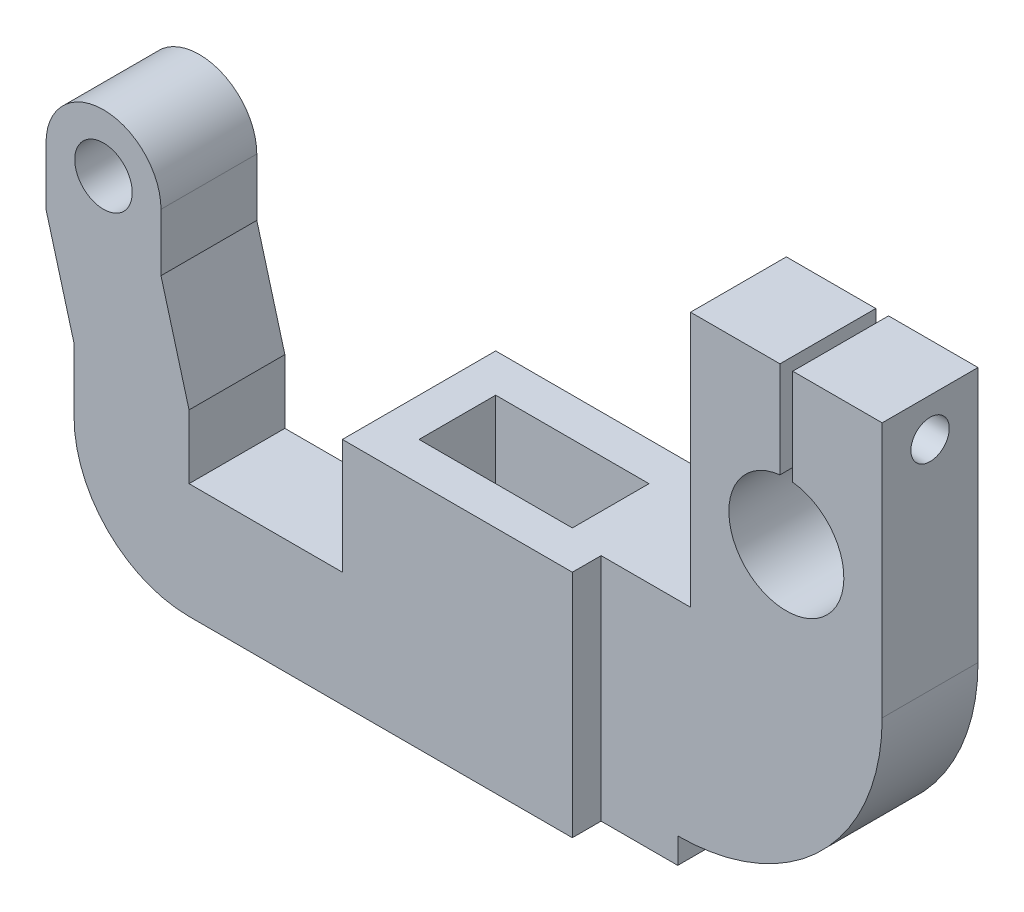
ISO-10303-21;
HEADER;
FILE_DESCRIPTION(('STEP AP214'),'2;1');
FILE_NAME('part.step','',(''),(''),'','','');
FILE_SCHEMA(('AUTOMOTIVE_DESIGN { 1 0 10303 214 1 1 1 1 }'));
ENDSEC;
DATA;
#1=APPLICATION_CONTEXT('core data for automotive mechanical design processes');
#2=APPLICATION_PROTOCOL_DEFINITION('international standard','automotive_design',2000,#1);
#3=PRODUCT_CONTEXT('',#1,'mechanical');
#4=PRODUCT('Part','Part','',(#3));
#5=PRODUCT_RELATED_PRODUCT_CATEGORY('part','',(#4));
#6=PRODUCT_DEFINITION_FORMATION('','',#4);
#7=PRODUCT_DEFINITION_CONTEXT('part definition',#1,'design');
#8=PRODUCT_DEFINITION('design','',#6,#7);
#9=PRODUCT_DEFINITION_SHAPE('','',#8);
#10=(LENGTH_UNIT() NAMED_UNIT(*) SI_UNIT(.MILLI.,.METRE.));
#11=(NAMED_UNIT(*) PLANE_ANGLE_UNIT() SI_UNIT($,.RADIAN.));
#12=(NAMED_UNIT(*) SI_UNIT($,.STERADIAN.) SOLID_ANGLE_UNIT());
#13=UNCERTAINTY_MEASURE_WITH_UNIT(LENGTH_MEASURE(1.E-05),#10,'distance_accuracy_value','');
#14=(GEOMETRIC_REPRESENTATION_CONTEXT(3) GLOBAL_UNCERTAINTY_ASSIGNED_CONTEXT((#13)) GLOBAL_UNIT_ASSIGNED_CONTEXT((#10,
#11,#12)) REPRESENTATION_CONTEXT('',''));
#15=CARTESIAN_POINT('',(0.,0.,0.));
#16=DIRECTION('',(0.,0.,1.));
#17=DIRECTION('',(1.,0.,0.));
#18=AXIS2_PLACEMENT_3D('',#15,#16,#17);
#19=CARTESIAN_POINT('',(-18.,36.,-12.));
#20=DIRECTION('',(1.,0.,0.));
#21=DIRECTION('',(0.,0.,-1.));
#22=AXIS2_PLACEMENT_3D('',#19,#20,#21);
#23=PLANE('',#22);
#24=DIRECTION('',(0.,0.,-1.));
#25=VECTOR('',#24,1.);
#26=CARTESIAN_POINT('',(-18.,18.,12.));
#27=LINE('',#26,#25);
#28=CARTESIAN_POINT('',(-18.,18.,12.));
#29=VERTEX_POINT('',#28);
#30=CARTESIAN_POINT('',(-18.,18.,-3.));
#31=VERTEX_POINT('',#30);
#32=EDGE_CURVE('E54',#29,#31,#27,.T.);
#33=ORIENTED_EDGE('',*,*,#32,.F.);
#34=DIRECTION('',(0.,-1.,0.));
#35=VECTOR('',#34,1.);
#36=CARTESIAN_POINT('',(-18.,36.,12.));
#37=LINE('',#36,#35);
#38=CARTESIAN_POINT('',(-18.,36.,12.));
#39=VERTEX_POINT('',#38);
#40=EDGE_CURVE('E480',#39,#29,#37,.T.);
#41=ORIENTED_EDGE('',*,*,#40,.F.);
#42=DIRECTION('',(0.,0.,1.));
#43=VECTOR('',#42,1.);
#44=CARTESIAN_POINT('',(-18.,36.,-12.));
#45=LINE('',#44,#43);
#46=CARTESIAN_POINT('',(-18.,36.,-12.));
#47=VERTEX_POINT('',#46);
#48=EDGE_CURVE('E459',#47,#39,#45,.T.);
#49=ORIENTED_EDGE('',*,*,#48,.F.);
#50=DIRECTION('',(0.,-1.,0.));
#51=VECTOR('',#50,1.);
#52=CARTESIAN_POINT('',(-18.,36.,-12.));
#53=LINE('',#52,#51);
#54=CARTESIAN_POINT('',(-18.,0.,-12.));
#55=VERTEX_POINT('',#54);
#56=EDGE_CURVE('E479',#47,#55,#53,.T.);
#57=ORIENTED_EDGE('',*,*,#56,.T.);
#58=DIRECTION('',(0.,0.,1.));
#59=VECTOR('',#58,1.);
#60=CARTESIAN_POINT('',(-18.,0.,-12.));
#61=LINE('',#60,#59);
#62=CARTESIAN_POINT('',(-18.,0.,-3.));
#63=VERTEX_POINT('',#62);
#64=EDGE_CURVE('E468',#55,#63,#61,.T.);
#65=ORIENTED_EDGE('',*,*,#64,.T.);
#66=DIRECTION('',(0.,1.,0.));
#67=VECTOR('',#66,1.);
#68=CARTESIAN_POINT('',(-18.,0.,-3.));
#69=LINE('',#68,#67);
#70=EDGE_CURVE('E324',#63,#31,#69,.T.);
#71=ORIENTED_EDGE('',*,*,#70,.T.);
#72=EDGE_LOOP('',(#33,#41,#49,#57,#65,#71));
#73=FACE_BOUND('',#72,.T.);
#74=ADVANCED_FACE('F39',(#73),#23,.F.);
#75=CARTESIAN_POINT('',(0.,76.,0.));
#76=DIRECTION('',(0.,-1.,0.));
#77=DIRECTION('',(0.,0.,-1.));
#78=AXIS2_PLACEMENT_3D('',#75,#76,#77);
#79=PLANE('',#78);
#80=DIRECTION('',(-1.,0.,0.));
#81=VECTOR('',#80,1.);
#82=CARTESIAN_POINT('',(62.,76.,-7.5));
#83=LINE('',#82,#81);
#84=CARTESIAN_POINT('',(62.,76.,-7.5));
#85=VERTEX_POINT('',#84);
#86=CARTESIAN_POINT('',(48.,76.,-7.5));
#87=VERTEX_POINT('',#86);
#88=EDGE_CURVE('E364',#85,#87,#83,.T.);
#89=ORIENTED_EDGE('',*,*,#88,.T.);
#90=DIRECTION('',(0.,0.,1.));
#91=VECTOR('',#90,1.);
#92=CARTESIAN_POINT('',(48.,76.,0.));
#93=LINE('',#92,#91);
#94=CARTESIAN_POINT('',(48.,76.,7.5));
#95=VERTEX_POINT('',#94);
#96=EDGE_CURVE('E11',#87,#95,#93,.T.);
#97=ORIENTED_EDGE('',*,*,#96,.T.);
#98=DIRECTION('',(1.,0.,0.));
#99=VECTOR('',#98,1.);
#100=CARTESIAN_POINT('',(62.,76.,7.5));
#101=LINE('',#100,#99);
#102=CARTESIAN_POINT('',(62.,76.,7.5));
#103=VERTEX_POINT('',#102);
#104=EDGE_CURVE('E367',#95,#103,#101,.T.);
#105=ORIENTED_EDGE('',*,*,#104,.T.);
#106=DIRECTION('',(0.,0.,-1.));
#107=VECTOR('',#106,1.);
#108=CARTESIAN_POINT('',(62.,76.,-7.5));
#109=LINE('',#108,#107);
#110=EDGE_CURVE('E359',#103,#85,#109,.T.);
#111=ORIENTED_EDGE('',*,*,#110,.T.);
#112=EDGE_LOOP('',(#89,#97,#105,#111));
#113=FACE_BOUND('',#112,.T.);
#114=ADVANCED_FACE('F512',(#113),#79,.F.);
#115=CARTESIAN_POINT('',(30.,0.,-7.5));
#116=DIRECTION('',(1.,0.,0.));
#117=DIRECTION('',(0.,0.,-1.));
#118=AXIS2_PLACEMENT_3D('',#115,#116,#117);
#119=PLANE('',#118);
#120=DIRECTION('',(0.,1.,0.));
#121=VECTOR('',#120,1.);
#122=CARTESIAN_POINT('',(30.,0.,-7.5));
#123=LINE('',#122,#121);
#124=CARTESIAN_POINT('',(30.,0.,-7.5));
#125=VERTEX_POINT('',#124);
#126=CARTESIAN_POINT('',(30.,4.,-7.5));
#127=VERTEX_POINT('',#126);
#128=EDGE_CURVE('E413',#125,#127,#123,.T.);
#129=ORIENTED_EDGE('',*,*,#128,.T.);
#130=DIRECTION('',(0.,0.,1.));
#131=VECTOR('',#130,1.);
#132=CARTESIAN_POINT('',(30.,4.,-7.5));
#133=LINE('',#132,#131);
#134=CARTESIAN_POINT('',(30.,4.,7.5));
#135=VERTEX_POINT('',#134);
#136=EDGE_CURVE('E388',#127,#135,#133,.T.);
#137=ORIENTED_EDGE('',*,*,#136,.T.);
#138=DIRECTION('',(0.,1.,0.));
#139=VECTOR('',#138,1.);
#140=CARTESIAN_POINT('',(30.,0.,7.5));
#141=LINE('',#140,#139);
#142=CARTESIAN_POINT('',(30.,0.,7.5));
#143=VERTEX_POINT('',#142);
#144=EDGE_CURVE('E419',#143,#135,#141,.T.);
#145=ORIENTED_EDGE('',*,*,#144,.F.);
#146=DIRECTION('',(0.,0.,-1.));
#147=VECTOR('',#146,1.);
#148=CARTESIAN_POINT('',(30.,0.,-7.5));
#149=LINE('',#148,#147);
#150=EDGE_CURVE('E402',#143,#125,#149,.T.);
#151=ORIENTED_EDGE('',*,*,#150,.T.);
#152=EDGE_LOOP('',(#129,#137,#145,#151));
#153=FACE_BOUND('',#152,.T.);
#154=ADVANCED_FACE('F525',(#153),#119,.T.);
#155=CARTESIAN_POINT('',(18.,36.,-12.));
#156=DIRECTION('',(-1.,0.,0.));
#157=DIRECTION('',(0.,0.,1.));
#158=AXIS2_PLACEMENT_3D('',#155,#156,#157);
#159=PLANE('',#158);
#160=DIRECTION('',(0.,1.,0.));
#161=VECTOR('',#160,1.);
#162=CARTESIAN_POINT('',(18.,0.,-7.5));
#163=LINE('',#162,#161);
#164=CARTESIAN_POINT('',(18.,0.,-7.5));
#165=VERTEX_POINT('',#164);
#166=CARTESIAN_POINT('',(18.,36.,-7.5));
#167=VERTEX_POINT('',#166);
#168=EDGE_CURVE('E408',#165,#167,#163,.T.);
#169=ORIENTED_EDGE('',*,*,#168,.F.);
#170=DIRECTION('',(0.,0.,-1.));
#171=VECTOR('',#170,1.);
#172=CARTESIAN_POINT('',(18.,0.,-12.));
#173=LINE('',#172,#171);
#174=CARTESIAN_POINT('',(18.,0.,-12.));
#175=VERTEX_POINT('',#174);
#176=EDGE_CURVE('E450',#165,#175,#173,.T.);
#177=ORIENTED_EDGE('',*,*,#176,.T.);
#178=DIRECTION('',(0.,-1.,0.));
#179=VECTOR('',#178,1.);
#180=CARTESIAN_POINT('',(18.,36.,-12.));
#181=LINE('',#180,#179);
#182=CARTESIAN_POINT('',(18.,36.,-12.));
#183=VERTEX_POINT('',#182);
#184=EDGE_CURVE('E482',#183,#175,#181,.T.);
#185=ORIENTED_EDGE('',*,*,#184,.F.);
#186=DIRECTION('',(0.,0.,-1.));
#187=VECTOR('',#186,1.);
#188=CARTESIAN_POINT('',(18.,36.,-12.));
#189=LINE('',#188,#187);
#190=EDGE_CURVE('E457',#167,#183,#189,.T.);
#191=ORIENTED_EDGE('',*,*,#190,.F.);
#192=EDGE_LOOP('',(#169,#177,#185,#191));
#193=FACE_BOUND('',#192,.T.);
#194=ADVANCED_FACE('F534',(#193),#159,.F.);
#195=CARTESIAN_POINT('',(18.,0.,12.));
#196=VERTEX_POINT('',#195);
#197=CARTESIAN_POINT('',(18.,0.,7.5));
#198=VERTEX_POINT('',#197);
#199=EDGE_CURVE('E461',#196,#198,#173,.T.);
#200=ORIENTED_EDGE('',*,*,#199,.T.);
#201=DIRECTION('',(0.,1.,0.));
#202=VECTOR('',#201,1.);
#203=CARTESIAN_POINT('',(18.,0.,7.5));
#204=LINE('',#203,#202);
#205=CARTESIAN_POINT('',(18.,36.,7.5));
#206=VERTEX_POINT('',#205);
#207=EDGE_CURVE('E410',#198,#206,#204,.T.);
#208=ORIENTED_EDGE('',*,*,#207,.T.);
#209=CARTESIAN_POINT('',(18.,36.,12.));
#210=VERTEX_POINT('',#209);
#211=EDGE_CURVE('E451',#210,#206,#189,.T.);
#212=ORIENTED_EDGE('',*,*,#211,.F.);
#213=DIRECTION('',(0.,-1.,0.));
#214=VECTOR('',#213,1.);
#215=CARTESIAN_POINT('',(18.,36.,12.));
#216=LINE('',#215,#214);
#217=EDGE_CURVE('E465',#210,#196,#216,.T.);
#218=ORIENTED_EDGE('',*,*,#217,.T.);
#219=EDGE_LOOP('',(#200,#208,#212,#218));
#220=FACE_BOUND('',#219,.T.);
#221=ADVANCED_FACE('F41',(#220),#159,.F.);
#222=CARTESIAN_POINT('',(-18.,36.,-12.));
#223=DIRECTION('',(0.,0.,1.));
#224=DIRECTION('',(1.,0.,0.));
#225=AXIS2_PLACEMENT_3D('',#222,#223,#224);
#226=PLANE('',#225);
#227=DIRECTION('',(-1.,0.,0.));
#228=VECTOR('',#227,1.);
#229=CARTESIAN_POINT('',(-18.,0.,-12.));
#230=LINE('',#229,#228);
#231=EDGE_CURVE('E466',#175,#55,#230,.T.);
#232=ORIENTED_EDGE('',*,*,#231,.T.);
#233=ORIENTED_EDGE('',*,*,#56,.F.);
#234=DIRECTION('',(-1.,0.,0.));
#235=VECTOR('',#234,1.);
#236=CARTESIAN_POINT('',(-18.,36.,-12.));
#237=LINE('',#236,#235);
#238=EDGE_CURVE('E460',#183,#47,#237,.T.);
#239=ORIENTED_EDGE('',*,*,#238,.F.);
#240=ORIENTED_EDGE('',*,*,#184,.T.);
#241=EDGE_LOOP('',(#232,#233,#239,#240));
#242=FACE_BOUND('',#241,.T.);
#243=ADVANCED_FACE('F545',(#242),#226,.F.);
#244=CARTESIAN_POINT('',(-18.,36.,12.));
#245=DIRECTION('',(0.,0.,-1.));
#246=DIRECTION('',(-1.,0.,0.));
#247=AXIS2_PLACEMENT_3D('',#244,#245,#246);
#248=PLANE('',#247);
#249=DIRECTION('',(1.,0.,0.));
#250=VECTOR('',#249,1.);
#251=CARTESIAN_POINT('',(-18.,0.,12.));
#252=LINE('',#251,#250);
#253=CARTESIAN_POINT('',(-42.,0.,12.));
#254=VERTEX_POINT('',#253);
#255=EDGE_CURVE('E474',#254,#196,#252,.T.);
#256=ORIENTED_EDGE('',*,*,#255,.T.);
#257=ORIENTED_EDGE('',*,*,#217,.F.);
#258=DIRECTION('',(1.,0.,0.));
#259=VECTOR('',#258,1.);
#260=CARTESIAN_POINT('',(-18.,36.,12.));
#261=LINE('',#260,#259);
#262=EDGE_CURVE('E464',#39,#210,#261,.T.);
#263=ORIENTED_EDGE('',*,*,#262,.F.);
#264=ORIENTED_EDGE('',*,*,#40,.T.);
#265=DIRECTION('',(1.,0.,0.));
#266=VECTOR('',#265,1.);
#267=CARTESIAN_POINT('',(-18.,18.,12.));
#268=LINE('',#267,#266);
#269=CARTESIAN_POINT('',(-42.,18.,12.));
#270=VERTEX_POINT('',#269);
#271=EDGE_CURVE('E322',#270,#29,#268,.T.);
#272=ORIENTED_EDGE('',*,*,#271,.F.);
#273=DIRECTION('',(0.,1.,0.));
#274=VECTOR('',#273,1.);
#275=CARTESIAN_POINT('',(-42.,18.,12.));
#276=LINE('',#275,#274);
#277=CARTESIAN_POINT('',(-42.,28.,12.));
#278=VERTEX_POINT('',#277);
#279=EDGE_CURVE('E293',#270,#278,#276,.T.);
#280=ORIENTED_EDGE('',*,*,#279,.T.);
#281=DIRECTION('',(-0.264769001023054,0.964311866616425,0.));
#282=VECTOR('',#281,1.);
#283=CARTESIAN_POINT('',(-42.,28.,12.));
#284=LINE('',#283,#282);
#285=CARTESIAN_POINT('',(-46.3930850205475,44.,12.));
#286=VERTEX_POINT('',#285);
#287=EDGE_CURVE('E282',#278,#286,#284,.T.);
#288=ORIENTED_EDGE('',*,*,#287,.T.);
#289=DIRECTION('',(0.,1.,0.));
#290=VECTOR('',#289,1.);
#291=CARTESIAN_POINT('',(-46.3930850205475,53.,12.));
#292=LINE('',#291,#290);
#293=CARTESIAN_POINT('',(-46.3930850205475,53.,12.));
#294=VERTEX_POINT('',#293);
#295=EDGE_CURVE('E274',#286,#294,#292,.T.);
#296=ORIENTED_EDGE('',*,*,#295,.T.);
#297=CARTESIAN_POINT('',(-55.3930850205475,53.,12.));
#298=DIRECTION('',(0.,0.,1.));
#299=DIRECTION('',(1.,0.,0.));
#300=AXIS2_PLACEMENT_3D('',#297,#298,#299);
#301=CIRCLE('',#300,9.);
#302=CARTESIAN_POINT('',(-64.3930850205475,53.,12.));
#303=VERTEX_POINT('',#302);
#304=EDGE_CURVE('E244',#294,#303,#301,.T.);
#305=ORIENTED_EDGE('',*,*,#304,.T.);
#306=DIRECTION('',(0.,-1.,0.));
#307=VECTOR('',#306,1.);
#308=CARTESIAN_POINT('',(-64.3930850205475,44.,12.));
#309=LINE('',#308,#307);
#310=CARTESIAN_POINT('',(-64.3930850205475,44.,12.));
#311=VERTEX_POINT('',#310);
#312=EDGE_CURVE('E264',#303,#311,#309,.T.);
#313=ORIENTED_EDGE('',*,*,#312,.T.);
#314=DIRECTION('',(0.264769001023054,-0.964311866616425,0.));
#315=VECTOR('',#314,1.);
#316=CARTESIAN_POINT('',(-60.,28.,12.));
#317=LINE('',#316,#315);
#318=CARTESIAN_POINT('',(-60.,28.,12.));
#319=VERTEX_POINT('',#318);
#320=EDGE_CURVE('E279',#311,#319,#317,.T.);
#321=ORIENTED_EDGE('',*,*,#320,.T.);
#322=DIRECTION('',(0.,-1.,0.));
#323=VECTOR('',#322,1.);
#324=CARTESIAN_POINT('',(-60.,18.,12.));
#325=LINE('',#324,#323);
#326=CARTESIAN_POINT('',(-60.,18.,12.));
#327=VERTEX_POINT('',#326);
#328=EDGE_CURVE('E304',#319,#327,#325,.T.);
#329=ORIENTED_EDGE('',*,*,#328,.T.);
#330=CARTESIAN_POINT('',(-42.,18.,12.));
#331=DIRECTION('',(0.,0.,1.));
#332=DIRECTION('',(1.,0.,0.));
#333=AXIS2_PLACEMENT_3D('',#330,#331,#332);
#334=CIRCLE('',#333,18.);
#335=EDGE_CURVE('E300',#327,#254,#334,.T.);
#336=ORIENTED_EDGE('',*,*,#335,.T.);
#337=EDGE_LOOP('',(#256,#257,#263,#264,#272,#280,#288,#296,#305,#313,#321,#329,#336));
#338=FACE_BOUND('',#337,.T.);
#339=CARTESIAN_POINT('',(-55.3930850205475,53.,12.));
#340=DIRECTION('',(0.,0.,1.));
#341=DIRECTION('',(1.,0.,0.));
#342=AXIS2_PLACEMENT_3D('',#339,#340,#341);
#343=CIRCLE('',#342,4.5);
#344=CARTESIAN_POINT('',(-50.8930850205475,53.,12.));
#345=VERTEX_POINT('',#344);
#346=EDGE_CURVE('E266',#345,#345,#343,.T.);
#347=ORIENTED_EDGE('',*,*,#346,.F.);
#348=EDGE_LOOP('',(#347));
#349=FACE_BOUND('',#348,.T.);
#350=ADVANCED_FACE('F553',(#338,#349),#248,.F.);
#351=CARTESIAN_POINT('',(0.,36.,0.));
#352=DIRECTION('',(0.,1.,0.));
#353=DIRECTION('',(0.,0.,1.));
#354=AXIS2_PLACEMENT_3D('',#351,#352,#353);
#355=PLANE('',#354);
#356=DIRECTION('',(0.,0.,1.));
#357=VECTOR('',#356,1.);
#358=CARTESIAN_POINT('',(32.,36.,-7.5));
#359=LINE('',#358,#357);
#360=CARTESIAN_POINT('',(32.,36.,-7.5));
#361=VERTEX_POINT('',#360);
#362=CARTESIAN_POINT('',(32.,36.,7.5));
#363=VERTEX_POINT('',#362);
#364=EDGE_CURVE('E360',#361,#363,#359,.T.);
#365=ORIENTED_EDGE('',*,*,#364,.F.);
#366=DIRECTION('',(-1.,0.,0.));
#367=VECTOR('',#366,1.);
#368=CARTESIAN_POINT('',(18.,36.,-7.5));
#369=LINE('',#368,#367);
#370=EDGE_CURVE('E405',#361,#167,#369,.T.);
#371=ORIENTED_EDGE('',*,*,#370,.T.);
#372=ORIENTED_EDGE('',*,*,#190,.T.);
#373=ORIENTED_EDGE('',*,*,#238,.T.);
#374=ORIENTED_EDGE('',*,*,#48,.T.);
#375=ORIENTED_EDGE('',*,*,#262,.T.);
#376=ORIENTED_EDGE('',*,*,#211,.T.);
#377=DIRECTION('',(1.,0.,0.));
#378=VECTOR('',#377,1.);
#379=CARTESIAN_POINT('',(18.,36.,7.5));
#380=LINE('',#379,#378);
#381=EDGE_CURVE('E394',#206,#363,#380,.T.);
#382=ORIENTED_EDGE('',*,*,#381,.T.);
#383=EDGE_LOOP('',(#365,#371,#372,#373,#374,#375,#376,#382));
#384=FACE_BOUND('',#383,.T.);
#385=DIRECTION('',(0.,0.,-1.));
#386=VECTOR('',#385,1.);
#387=CARTESIAN_POINT('',(12.,36.,-6.));
#388=LINE('',#387,#386);
#389=CARTESIAN_POINT('',(12.,36.,6.));
#390=VERTEX_POINT('',#389);
#391=CARTESIAN_POINT('',(12.,36.,-6.));
#392=VERTEX_POINT('',#391);
#393=EDGE_CURVE('E412',#390,#392,#388,.T.);
#394=ORIENTED_EDGE('',*,*,#393,.F.);
#395=DIRECTION('',(1.,0.,0.));
#396=VECTOR('',#395,1.);
#397=CARTESIAN_POINT('',(-12.,36.,6.));
#398=LINE('',#397,#396);
#399=CARTESIAN_POINT('',(-12.,36.,6.));
#400=VERTEX_POINT('',#399);
#401=EDGE_CURVE('E428',#400,#390,#398,.T.);
#402=ORIENTED_EDGE('',*,*,#401,.F.);
#403=DIRECTION('',(0.,0.,1.));
#404=VECTOR('',#403,1.);
#405=CARTESIAN_POINT('',(-12.,36.,-6.));
#406=LINE('',#405,#404);
#407=CARTESIAN_POINT('',(-12.,36.,-6.));
#408=VERTEX_POINT('',#407);
#409=EDGE_CURVE('E439',#408,#400,#406,.T.);
#410=ORIENTED_EDGE('',*,*,#409,.F.);
#411=DIRECTION('',(-1.,0.,0.));
#412=VECTOR('',#411,1.);
#413=CARTESIAN_POINT('',(-12.,36.,-6.));
#414=LINE('',#413,#412);
#415=EDGE_CURVE('E440',#392,#408,#414,.T.);
#416=ORIENTED_EDGE('',*,*,#415,.F.);
#417=EDGE_LOOP('',(#394,#402,#410,#416));
#418=FACE_BOUND('',#417,.T.);
#419=ADVANCED_FACE('F539',(#384,#418),#355,.T.);
#420=CARTESIAN_POINT('',(0.,0.,0.));
#421=DIRECTION('',(0.,1.,0.));
#422=DIRECTION('',(0.,0.,1.));
#423=AXIS2_PLACEMENT_3D('',#420,#421,#422);
#424=PLANE('',#423);
#425=DIRECTION('',(1.,0.,0.));
#426=VECTOR('',#425,1.);
#427=CARTESIAN_POINT('',(-12.,0.,6.));
#428=LINE('',#427,#426);
#429=CARTESIAN_POINT('',(-12.,0.,6.));
#430=VERTEX_POINT('',#429);
#431=CARTESIAN_POINT('',(12.,0.,6.));
#432=VERTEX_POINT('',#431);
#433=EDGE_CURVE('E435',#430,#432,#428,.T.);
#434=ORIENTED_EDGE('',*,*,#433,.T.);
#435=DIRECTION('',(0.,0.,-1.));
#436=VECTOR('',#435,1.);
#437=CARTESIAN_POINT('',(12.,0.,-6.));
#438=LINE('',#437,#436);
#439=CARTESIAN_POINT('',(12.,0.,-6.));
#440=VERTEX_POINT('',#439);
#441=EDGE_CURVE('E422',#432,#440,#438,.T.);
#442=ORIENTED_EDGE('',*,*,#441,.T.);
#443=DIRECTION('',(-1.,0.,0.));
#444=VECTOR('',#443,1.);
#445=CARTESIAN_POINT('',(-12.,0.,-6.));
#446=LINE('',#445,#444);
#447=CARTESIAN_POINT('',(-12.,0.,-6.));
#448=VERTEX_POINT('',#447);
#449=EDGE_CURVE('E424',#440,#448,#446,.T.);
#450=ORIENTED_EDGE('',*,*,#449,.T.);
#451=DIRECTION('',(0.,0.,1.));
#452=VECTOR('',#451,1.);
#453=CARTESIAN_POINT('',(-12.,0.,-6.));
#454=LINE('',#453,#452);
#455=EDGE_CURVE('E429',#448,#430,#454,.T.);
#456=ORIENTED_EDGE('',*,*,#455,.T.);
#457=EDGE_LOOP('',(#434,#442,#450,#456));
#458=FACE_BOUND('',#457,.T.);
#459=ORIENTED_EDGE('',*,*,#199,.F.);
#460=ORIENTED_EDGE('',*,*,#255,.F.);
#461=DIRECTION('',(0.,0.,1.));
#462=VECTOR('',#461,1.);
#463=CARTESIAN_POINT('',(-42.,0.,12.));
#464=LINE('',#463,#462);
#465=CARTESIAN_POINT('',(-42.,0.,-3.));
#466=VERTEX_POINT('',#465);
#467=EDGE_CURVE('E318',#466,#254,#464,.T.);
#468=ORIENTED_EDGE('',*,*,#467,.F.);
#469=DIRECTION('',(-1.,0.,0.));
#470=VECTOR('',#469,1.);
#471=CARTESIAN_POINT('',(-18.,0.,-3.));
#472=LINE('',#471,#470);
#473=EDGE_CURVE('E320',#63,#466,#472,.T.);
#474=ORIENTED_EDGE('',*,*,#473,.F.);
#475=ORIENTED_EDGE('',*,*,#64,.F.);
#476=ORIENTED_EDGE('',*,*,#231,.F.);
#477=ORIENTED_EDGE('',*,*,#176,.F.);
#478=DIRECTION('',(-1.,0.,0.));
#479=VECTOR('',#478,1.);
#480=CARTESIAN_POINT('',(18.,0.,-7.5));
#481=LINE('',#480,#479);
#482=EDGE_CURVE('E403',#125,#165,#481,.T.);
#483=ORIENTED_EDGE('',*,*,#482,.F.);
#484=ORIENTED_EDGE('',*,*,#150,.F.);
#485=DIRECTION('',(1.,0.,0.));
#486=VECTOR('',#485,1.);
#487=CARTESIAN_POINT('',(18.,0.,7.5));
#488=LINE('',#487,#486);
#489=EDGE_CURVE('E397',#198,#143,#488,.T.);
#490=ORIENTED_EDGE('',*,*,#489,.F.);
#491=EDGE_LOOP('',(#459,#460,#468,#474,#475,#476,#477,#483,#484,#490));
#492=FACE_BOUND('',#491,.T.);
#493=ADVANCED_FACE('F530',(#458,#492),#424,.F.);
#494=CARTESIAN_POINT('',(12.,0.,-6.));
#495=DIRECTION('',(1.,0.,0.));
#496=DIRECTION('',(0.,0.,-1.));
#497=AXIS2_PLACEMENT_3D('',#494,#495,#496);
#498=PLANE('',#497);
#499=ORIENTED_EDGE('',*,*,#393,.T.);
#500=DIRECTION('',(0.,1.,0.));
#501=VECTOR('',#500,1.);
#502=CARTESIAN_POINT('',(12.,0.,-6.));
#503=LINE('',#502,#501);
#504=EDGE_CURVE('E434',#440,#392,#503,.T.);
#505=ORIENTED_EDGE('',*,*,#504,.F.);
#506=ORIENTED_EDGE('',*,*,#441,.F.);
#507=DIRECTION('',(0.,1.,0.));
#508=VECTOR('',#507,1.);
#509=CARTESIAN_POINT('',(12.,0.,6.));
#510=LINE('',#509,#508);
#511=EDGE_CURVE('E444',#432,#390,#510,.T.);
#512=ORIENTED_EDGE('',*,*,#511,.T.);
#513=EDGE_LOOP('',(#499,#505,#506,#512));
#514=FACE_BOUND('',#513,.T.);
#515=ADVANCED_FACE('F622',(#514),#498,.F.);
#516=CARTESIAN_POINT('',(-12.,0.,6.));
#517=DIRECTION('',(0.,0.,1.));
#518=DIRECTION('',(1.,0.,0.));
#519=AXIS2_PLACEMENT_3D('',#516,#517,#518);
#520=PLANE('',#519);
#521=ORIENTED_EDGE('',*,*,#401,.T.);
#522=ORIENTED_EDGE('',*,*,#511,.F.);
#523=ORIENTED_EDGE('',*,*,#433,.F.);
#524=DIRECTION('',(0.,1.,0.));
#525=VECTOR('',#524,1.);
#526=CARTESIAN_POINT('',(-12.,0.,6.));
#527=LINE('',#526,#525);
#528=EDGE_CURVE('E449',#430,#400,#527,.T.);
#529=ORIENTED_EDGE('',*,*,#528,.T.);
#530=EDGE_LOOP('',(#521,#522,#523,#529));
#531=FACE_BOUND('',#530,.T.);
#532=ADVANCED_FACE('F623',(#531),#520,.F.);
#533=CARTESIAN_POINT('',(-12.,0.,-6.));
#534=DIRECTION('',(-1.,0.,0.));
#535=DIRECTION('',(0.,0.,1.));
#536=AXIS2_PLACEMENT_3D('',#533,#534,#535);
#537=PLANE('',#536);
#538=ORIENTED_EDGE('',*,*,#409,.T.);
#539=ORIENTED_EDGE('',*,*,#528,.F.);
#540=ORIENTED_EDGE('',*,*,#455,.F.);
#541=DIRECTION('',(0.,1.,0.));
#542=VECTOR('',#541,1.);
#543=CARTESIAN_POINT('',(-12.,0.,-6.));
#544=LINE('',#543,#542);
#545=EDGE_CURVE('E448',#448,#408,#544,.T.);
#546=ORIENTED_EDGE('',*,*,#545,.T.);
#547=EDGE_LOOP('',(#538,#539,#540,#546));
#548=FACE_BOUND('',#547,.T.);
#549=ADVANCED_FACE('F624',(#548),#537,.F.);
#550=CARTESIAN_POINT('',(-12.,0.,-6.));
#551=DIRECTION('',(0.,0.,-1.));
#552=DIRECTION('',(-1.,0.,0.));
#553=AXIS2_PLACEMENT_3D('',#550,#551,#552);
#554=PLANE('',#553);
#555=ORIENTED_EDGE('',*,*,#415,.T.);
#556=ORIENTED_EDGE('',*,*,#545,.F.);
#557=ORIENTED_EDGE('',*,*,#449,.F.);
#558=ORIENTED_EDGE('',*,*,#504,.T.);
#559=EDGE_LOOP('',(#555,#556,#557,#558));
#560=FACE_BOUND('',#559,.T.);
#561=ADVANCED_FACE('F627',(#560),#554,.F.);
#562=CARTESIAN_POINT('',(18.,0.,-7.5));
#563=DIRECTION('',(0.,0.,-1.));
#564=DIRECTION('',(-1.,0.,0.));
#565=AXIS2_PLACEMENT_3D('',#562,#563,#564);
#566=PLANE('',#565);
#567=DIRECTION('',(0.,-1.,0.));
#568=VECTOR('',#567,1.);
#569=CARTESIAN_POINT('',(48.,0.,-7.5));
#570=LINE('',#569,#568);
#571=CARTESIAN_POINT('',(48.,60.9442719099992,-7.5));
#572=VERTEX_POINT('',#571);
#573=EDGE_CURVE('E351',#87,#572,#570,.T.);
#574=ORIENTED_EDGE('',*,*,#573,.F.);
#575=ORIENTED_EDGE('',*,*,#88,.F.);
#576=DIRECTION('',(0.,-1.,0.));
#577=VECTOR('',#576,1.);
#578=CARTESIAN_POINT('',(62.,76.,-7.5));
#579=LINE('',#578,#577);
#580=CARTESIAN_POINT('',(62.,36.,-7.5));
#581=VERTEX_POINT('',#580);
#582=EDGE_CURVE('E381',#85,#581,#579,.T.);
#583=ORIENTED_EDGE('',*,*,#582,.T.);
#584=CARTESIAN_POINT('',(30.,36.,-7.5));
#585=DIRECTION('',(0.,0.,1.));
#586=DIRECTION('',(1.,0.,0.));
#587=AXIS2_PLACEMENT_3D('',#584,#585,#586);
#588=CIRCLE('',#587,32.);
#589=EDGE_CURVE('E389',#127,#581,#588,.T.);
#590=ORIENTED_EDGE('',*,*,#589,.F.);
#591=ORIENTED_EDGE('',*,*,#128,.F.);
#592=ORIENTED_EDGE('',*,*,#482,.T.);
#593=ORIENTED_EDGE('',*,*,#168,.T.);
#594=ORIENTED_EDGE('',*,*,#370,.F.);
#595=DIRECTION('',(0.,-1.,0.));
#596=VECTOR('',#595,1.);
#597=CARTESIAN_POINT('',(32.,76.,-7.5));
#598=LINE('',#597,#596);
#599=CARTESIAN_POINT('',(32.,76.,-7.5));
#600=VERTEX_POINT('',#599);
#601=EDGE_CURVE('E382',#600,#361,#598,.T.);
#602=ORIENTED_EDGE('',*,*,#601,.F.);
#603=CARTESIAN_POINT('',(46.,76.,-7.5));
#604=VERTEX_POINT('',#603);
#605=EDGE_CURVE('E361',#604,#600,#83,.T.);
#606=ORIENTED_EDGE('',*,*,#605,.F.);
#607=DIRECTION('',(0.,1.,0.));
#608=VECTOR('',#607,1.);
#609=CARTESIAN_POINT('',(46.,0.,-7.5));
#610=LINE('',#609,#608);
#611=CARTESIAN_POINT('',(46.,60.9442719099992,-7.5));
#612=VERTEX_POINT('',#611);
#613=EDGE_CURVE('E64',#612,#604,#610,.T.);
#614=ORIENTED_EDGE('',*,*,#613,.F.);
#615=CARTESIAN_POINT('',(47.,52.,-7.5));
#616=DIRECTION('',(0.,0.,-1.));
#617=DIRECTION('',(-1.,0.,0.));
#618=AXIS2_PLACEMENT_3D('',#615,#616,#617);
#619=CIRCLE('',#618,9.00000000000001);
#620=EDGE_CURVE('E357',#572,#612,#619,.T.);
#621=ORIENTED_EDGE('',*,*,#620,.F.);
#622=EDGE_LOOP('',(#574,#575,#583,#590,#591,#592,#593,#594,#602,#606,#614,#621));
#623=FACE_BOUND('',#622,.T.);
#624=ADVANCED_FACE('F494',(#623),#566,.T.);
#625=CARTESIAN_POINT('',(18.,0.,7.5));
#626=DIRECTION('',(0.,0.,1.));
#627=DIRECTION('',(1.,0.,0.));
#628=AXIS2_PLACEMENT_3D('',#625,#626,#627);
#629=PLANE('',#628);
#630=DIRECTION('',(0.,1.,0.));
#631=VECTOR('',#630,1.);
#632=CARTESIAN_POINT('',(48.,76.,7.5));
#633=LINE('',#632,#631);
#634=CARTESIAN_POINT('',(48.,60.9442719099992,7.5));
#635=VERTEX_POINT('',#634);
#636=EDGE_CURVE('E347',#635,#95,#633,.T.);
#637=ORIENTED_EDGE('',*,*,#636,.F.);
#638=CARTESIAN_POINT('',(47.,52.,7.5));
#639=DIRECTION('',(0.,0.,1.));
#640=DIRECTION('',(1.,0.,0.));
#641=AXIS2_PLACEMENT_3D('',#638,#639,#640);
#642=CIRCLE('',#641,9.00000000000001);
#643=CARTESIAN_POINT('',(46.,60.9442719099992,7.5));
#644=VERTEX_POINT('',#643);
#645=EDGE_CURVE('E343',#644,#635,#642,.T.);
#646=ORIENTED_EDGE('',*,*,#645,.F.);
#647=DIRECTION('',(0.,-1.,0.));
#648=VECTOR('',#647,1.);
#649=CARTESIAN_POINT('',(46.,76.,7.5));
#650=LINE('',#649,#648);
#651=CARTESIAN_POINT('',(46.,76.,7.5));
#652=VERTEX_POINT('',#651);
#653=EDGE_CURVE('E345',#652,#644,#650,.T.);
#654=ORIENTED_EDGE('',*,*,#653,.F.);
#655=CARTESIAN_POINT('',(32.,76.,7.5));
#656=VERTEX_POINT('',#655);
#657=EDGE_CURVE('E369',#656,#652,#101,.T.);
#658=ORIENTED_EDGE('',*,*,#657,.F.);
#659=DIRECTION('',(0.,-1.,0.));
#660=VECTOR('',#659,1.);
#661=CARTESIAN_POINT('',(32.,76.,7.5));
#662=LINE('',#661,#660);
#663=EDGE_CURVE('E377',#656,#363,#662,.T.);
#664=ORIENTED_EDGE('',*,*,#663,.T.);
#665=ORIENTED_EDGE('',*,*,#381,.F.);
#666=ORIENTED_EDGE('',*,*,#207,.F.);
#667=ORIENTED_EDGE('',*,*,#489,.T.);
#668=ORIENTED_EDGE('',*,*,#144,.T.);
#669=CARTESIAN_POINT('',(30.,36.,7.5));
#670=DIRECTION('',(0.,0.,1.));
#671=DIRECTION('',(1.,0.,0.));
#672=AXIS2_PLACEMENT_3D('',#669,#670,#671);
#673=CIRCLE('',#672,32.);
#674=CARTESIAN_POINT('',(62.,36.,7.5));
#675=VERTEX_POINT('',#674);
#676=EDGE_CURVE('E390',#135,#675,#673,.T.);
#677=ORIENTED_EDGE('',*,*,#676,.T.);
#678=DIRECTION('',(0.,-1.,0.));
#679=VECTOR('',#678,1.);
#680=CARTESIAN_POINT('',(62.,76.,7.5));
#681=LINE('',#680,#679);
#682=EDGE_CURVE('E373',#103,#675,#681,.T.);
#683=ORIENTED_EDGE('',*,*,#682,.F.);
#684=ORIENTED_EDGE('',*,*,#104,.F.);
#685=EDGE_LOOP('',(#637,#646,#654,#658,#664,#665,#666,#667,#668,#677,#683,#684));
#686=FACE_BOUND('',#685,.T.);
#687=ADVANCED_FACE('F503',(#686),#629,.T.);
#688=CARTESIAN_POINT('',(30.,36.,-7.5));
#689=DIRECTION('',(0.,0.,1.));
#690=DIRECTION('',(1.,0.,0.));
#691=AXIS2_PLACEMENT_3D('',#688,#689,#690);
#692=CYLINDRICAL_SURFACE('',#691,32.);
#693=ORIENTED_EDGE('',*,*,#676,.F.);
#694=ORIENTED_EDGE('',*,*,#136,.F.);
#695=ORIENTED_EDGE('',*,*,#589,.T.);
#696=DIRECTION('',(0.,0.,1.));
#697=VECTOR('',#696,1.);
#698=CARTESIAN_POINT('',(62.,36.,-7.5));
#699=LINE('',#698,#697);
#700=EDGE_CURVE('E392',#581,#675,#699,.T.);
#701=ORIENTED_EDGE('',*,*,#700,.T.);
#702=EDGE_LOOP('',(#693,#694,#695,#701));
#703=FACE_BOUND('',#702,.T.);
#704=ADVANCED_FACE('F619',(#703),#692,.T.);
#705=CARTESIAN_POINT('',(62.,76.,-7.5));
#706=DIRECTION('',(-1.,0.,0.));
#707=DIRECTION('',(0.,0.,1.));
#708=AXIS2_PLACEMENT_3D('',#705,#706,#707);
#709=PLANE('',#708);
#710=CARTESIAN_POINT('',(62.,70.,0.));
#711=DIRECTION('',(1.,0.,0.));
#712=DIRECTION('',(0.,0.,-1.));
#713=AXIS2_PLACEMENT_3D('',#710,#711,#712);
#714=CIRCLE('',#713,3.);
#715=CARTESIAN_POINT('',(62.,70.,-3.));
#716=VERTEX_POINT('',#715);
#717=EDGE_CURVE('E332',#716,#716,#714,.T.);
#718=ORIENTED_EDGE('',*,*,#717,.F.);
#719=EDGE_LOOP('',(#718));
#720=FACE_BOUND('',#719,.T.);
#721=ORIENTED_EDGE('',*,*,#700,.F.);
#722=ORIENTED_EDGE('',*,*,#582,.F.);
#723=ORIENTED_EDGE('',*,*,#110,.F.);
#724=ORIENTED_EDGE('',*,*,#682,.T.);
#725=EDGE_LOOP('',(#721,#722,#723,#724));
#726=FACE_BOUND('',#725,.T.);
#727=ADVANCED_FACE('F519',(#720,#726),#709,.F.);
#728=CARTESIAN_POINT('',(32.,76.,-7.5));
#729=DIRECTION('',(1.,0.,0.));
#730=DIRECTION('',(0.,0.,-1.));
#731=AXIS2_PLACEMENT_3D('',#728,#729,#730);
#732=PLANE('',#731);
#733=CARTESIAN_POINT('',(32.,70.,0.));
#734=DIRECTION('',(1.,0.,0.));
#735=DIRECTION('',(0.,0.,-1.));
#736=AXIS2_PLACEMENT_3D('',#733,#734,#735);
#737=CIRCLE('',#736,3.);
#738=CARTESIAN_POINT('',(32.,70.,-3.));
#739=VERTEX_POINT('',#738);
#740=EDGE_CURVE('E339',#739,#739,#737,.T.);
#741=ORIENTED_EDGE('',*,*,#740,.T.);
#742=EDGE_LOOP('',(#741));
#743=FACE_BOUND('',#742,.T.);
#744=ORIENTED_EDGE('',*,*,#364,.T.);
#745=ORIENTED_EDGE('',*,*,#663,.F.);
#746=DIRECTION('',(0.,0.,1.));
#747=VECTOR('',#746,1.);
#748=CARTESIAN_POINT('',(32.,76.,-7.5));
#749=LINE('',#748,#747);
#750=EDGE_CURVE('E370',#600,#656,#749,.T.);
#751=ORIENTED_EDGE('',*,*,#750,.F.);
#752=ORIENTED_EDGE('',*,*,#601,.T.);
#753=EDGE_LOOP('',(#744,#745,#751,#752));
#754=FACE_BOUND('',#753,.T.);
#755=ADVANCED_FACE('F499',(#743,#754),#732,.F.);
#756=ORIENTED_EDGE('',*,*,#657,.T.);
#757=DIRECTION('',(0.,0.,-1.));
#758=VECTOR('',#757,1.);
#759=CARTESIAN_POINT('',(46.,76.,0.));
#760=LINE('',#759,#758);
#761=EDGE_CURVE('E48',#652,#604,#760,.T.);
#762=ORIENTED_EDGE('',*,*,#761,.T.);
#763=ORIENTED_EDGE('',*,*,#605,.T.);
#764=ORIENTED_EDGE('',*,*,#750,.T.);
#765=EDGE_LOOP('',(#756,#762,#763,#764));
#766=FACE_BOUND('',#765,.T.);
#767=ADVANCED_FACE('F486',(#766),#79,.F.);
#768=CARTESIAN_POINT('',(48.,76.,-12.));
#769=DIRECTION('',(1.,0.,0.));
#770=DIRECTION('',(0.,0.,-1.));
#771=AXIS2_PLACEMENT_3D('',#768,#769,#770);
#772=PLANE('',#771);
#773=CARTESIAN_POINT('',(48.,70.,0.));
#774=DIRECTION('',(1.,0.,0.));
#775=DIRECTION('',(0.,0.,-1.));
#776=AXIS2_PLACEMENT_3D('',#773,#774,#775);
#777=CIRCLE('',#776,3.);
#778=CARTESIAN_POINT('',(48.,70.,-3.));
#779=VERTEX_POINT('',#778);
#780=EDGE_CURVE('E337',#779,#779,#777,.T.);
#781=ORIENTED_EDGE('',*,*,#780,.T.);
#782=EDGE_LOOP('',(#781));
#783=FACE_BOUND('',#782,.T.);
#784=ORIENTED_EDGE('',*,*,#573,.T.);
#785=DIRECTION('',(0.,0.,1.));
#786=VECTOR('',#785,1.);
#787=CARTESIAN_POINT('',(48.,60.9442719099992,-12.));
#788=LINE('',#787,#786);
#789=EDGE_CURVE('E353',#572,#635,#788,.T.);
#790=ORIENTED_EDGE('',*,*,#789,.T.);
#791=ORIENTED_EDGE('',*,*,#636,.T.);
#792=ORIENTED_EDGE('',*,*,#96,.F.);
#793=EDGE_LOOP('',(#784,#790,#791,#792));
#794=FACE_BOUND('',#793,.T.);
#795=ADVANCED_FACE('F770',(#783,#794),#772,.F.);
#796=CARTESIAN_POINT('',(47.,52.,-12.));
#797=DIRECTION('',(0.,0.,1.));
#798=DIRECTION('',(1.,0.,0.));
#799=AXIS2_PLACEMENT_3D('',#796,#797,#798);
#800=CYLINDRICAL_SURFACE('',#799,9.00000000000001);
#801=ORIENTED_EDGE('',*,*,#620,.T.);
#802=DIRECTION('',(0.,0.,1.));
#803=VECTOR('',#802,1.);
#804=CARTESIAN_POINT('',(46.,60.9442719099992,-12.));
#805=LINE('',#804,#803);
#806=EDGE_CURVE('E349',#612,#644,#805,.T.);
#807=ORIENTED_EDGE('',*,*,#806,.T.);
#808=ORIENTED_EDGE('',*,*,#645,.T.);
#809=ORIENTED_EDGE('',*,*,#789,.F.);
#810=EDGE_LOOP('',(#801,#807,#808,#809));
#811=FACE_BOUND('',#810,.T.);
#812=ADVANCED_FACE('F510',(#811),#800,.F.);
#813=CARTESIAN_POINT('',(46.,76.,-12.));
#814=DIRECTION('',(-1.,0.,0.));
#815=DIRECTION('',(0.,0.,1.));
#816=AXIS2_PLACEMENT_3D('',#813,#814,#815);
#817=PLANE('',#816);
#818=CARTESIAN_POINT('',(46.,70.,0.));
#819=DIRECTION('',(-1.,0.,0.));
#820=DIRECTION('',(0.,0.,1.));
#821=AXIS2_PLACEMENT_3D('',#818,#819,#820);
#822=CIRCLE('',#821,3.);
#823=CARTESIAN_POINT('',(46.,70.,3.));
#824=VERTEX_POINT('',#823);
#825=EDGE_CURVE('E43',#824,#824,#822,.T.);
#826=ORIENTED_EDGE('',*,*,#825,.T.);
#827=EDGE_LOOP('',(#826));
#828=FACE_BOUND('',#827,.T.);
#829=ORIENTED_EDGE('',*,*,#613,.T.);
#830=ORIENTED_EDGE('',*,*,#761,.F.);
#831=ORIENTED_EDGE('',*,*,#653,.T.);
#832=ORIENTED_EDGE('',*,*,#806,.F.);
#833=EDGE_LOOP('',(#829,#830,#831,#832));
#834=FACE_BOUND('',#833,.T.);
#835=ADVANCED_FACE('F504',(#828,#834),#817,.F.);
#836=CARTESIAN_POINT('',(-18.,70.,0.));
#837=DIRECTION('',(1.,0.,0.));
#838=DIRECTION('',(0.,0.,-1.));
#839=AXIS2_PLACEMENT_3D('',#836,#837,#838);
#840=CYLINDRICAL_SURFACE('',#839,3.);
#841=ORIENTED_EDGE('',*,*,#825,.F.);
#842=EDGE_LOOP('',(#841));
#843=FACE_BOUND('',#842,.T.);
#844=ORIENTED_EDGE('',*,*,#740,.F.);
#845=EDGE_LOOP('',(#844));
#846=FACE_BOUND('',#845,.T.);
#847=ADVANCED_FACE('F761',(#843,#846),#840,.F.);
#848=ORIENTED_EDGE('',*,*,#717,.T.);
#849=EDGE_LOOP('',(#848));
#850=FACE_BOUND('',#849,.T.);
#851=ORIENTED_EDGE('',*,*,#780,.F.);
#852=EDGE_LOOP('',(#851));
#853=FACE_BOUND('',#852,.T.);
#854=ADVANCED_FACE('F676',(#850,#853),#840,.F.);
#855=CARTESIAN_POINT('',(-18.,0.,-3.));
#856=DIRECTION('',(0.,0.,-1.));
#857=DIRECTION('',(-1.,0.,0.));
#858=AXIS2_PLACEMENT_3D('',#855,#856,#857);
#859=PLANE('',#858);
#860=DIRECTION('',(-1.,0.,0.));
#861=VECTOR('',#860,1.);
#862=CARTESIAN_POINT('',(-18.,18.,-3.));
#863=LINE('',#862,#861);
#864=CARTESIAN_POINT('',(-42.,18.,-3.));
#865=VERTEX_POINT('',#864);
#866=EDGE_CURVE('E323',#31,#865,#863,.T.);
#867=ORIENTED_EDGE('',*,*,#866,.F.);
#868=ORIENTED_EDGE('',*,*,#70,.F.);
#869=ORIENTED_EDGE('',*,*,#473,.T.);
#870=CARTESIAN_POINT('',(-42.,18.,-3.));
#871=DIRECTION('',(0.,0.,1.));
#872=DIRECTION('',(1.,0.,0.));
#873=AXIS2_PLACEMENT_3D('',#870,#871,#872);
#874=CIRCLE('',#873,18.);
#875=CARTESIAN_POINT('',(-60.,18.,-3.));
#876=VERTEX_POINT('',#875);
#877=EDGE_CURVE('E297',#876,#466,#874,.T.);
#878=ORIENTED_EDGE('',*,*,#877,.F.);
#879=DIRECTION('',(0.,-1.,0.));
#880=VECTOR('',#879,1.);
#881=CARTESIAN_POINT('',(-60.,18.,-3.));
#882=LINE('',#881,#880);
#883=CARTESIAN_POINT('',(-60.,28.,-3.));
#884=VERTEX_POINT('',#883);
#885=EDGE_CURVE('E298',#884,#876,#882,.T.);
#886=ORIENTED_EDGE('',*,*,#885,.F.);
#887=DIRECTION('',(0.264769001023054,-0.964311866616425,0.));
#888=VECTOR('',#887,1.);
#889=CARTESIAN_POINT('',(-60.,28.,-3.));
#890=LINE('',#889,#888);
#891=CARTESIAN_POINT('',(-64.3930850205475,44.,-3.));
#892=VERTEX_POINT('',#891);
#893=EDGE_CURVE('E278',#892,#884,#890,.T.);
#894=ORIENTED_EDGE('',*,*,#893,.F.);
#895=DIRECTION('',(0.,-1.,0.));
#896=VECTOR('',#895,1.);
#897=CARTESIAN_POINT('',(-64.3930850205475,44.,-3.));
#898=LINE('',#897,#896);
#899=CARTESIAN_POINT('',(-64.3930850205475,53.,-3.));
#900=VERTEX_POINT('',#899);
#901=EDGE_CURVE('E252',#900,#892,#898,.T.);
#902=ORIENTED_EDGE('',*,*,#901,.F.);
#903=CARTESIAN_POINT('',(-55.3930850205475,53.,-3.));
#904=DIRECTION('',(0.,0.,1.));
#905=DIRECTION('',(1.,0.,0.));
#906=AXIS2_PLACEMENT_3D('',#903,#904,#905);
#907=CIRCLE('',#906,9.);
#908=CARTESIAN_POINT('',(-46.3930850205475,53.,-3.));
#909=VERTEX_POINT('',#908);
#910=EDGE_CURVE('E245',#909,#900,#907,.T.);
#911=ORIENTED_EDGE('',*,*,#910,.F.);
#912=DIRECTION('',(0.,1.,0.));
#913=VECTOR('',#912,1.);
#914=CARTESIAN_POINT('',(-46.3930850205475,53.,-3.));
#915=LINE('',#914,#913);
#916=CARTESIAN_POINT('',(-46.3930850205475,44.,-3.));
#917=VERTEX_POINT('',#916);
#918=EDGE_CURVE('E259',#917,#909,#915,.T.);
#919=ORIENTED_EDGE('',*,*,#918,.F.);
#920=DIRECTION('',(-0.264769001023054,0.964311866616425,0.));
#921=VECTOR('',#920,1.);
#922=CARTESIAN_POINT('',(-42.,28.,-3.));
#923=LINE('',#922,#921);
#924=CARTESIAN_POINT('',(-42.,28.,-3.));
#925=VERTEX_POINT('',#924);
#926=EDGE_CURVE('E285',#925,#917,#923,.T.);
#927=ORIENTED_EDGE('',*,*,#926,.F.);
#928=DIRECTION('',(0.,1.,0.));
#929=VECTOR('',#928,1.);
#930=CARTESIAN_POINT('',(-42.,0.,-3.));
#931=LINE('',#930,#929);
#932=EDGE_CURVE('E291',#865,#925,#931,.T.);
#933=ORIENTED_EDGE('',*,*,#932,.F.);
#934=EDGE_LOOP('',(#867,#868,#869,#878,#886,#894,#902,#911,#919,#927,#933));
#935=FACE_BOUND('',#934,.T.);
#936=CARTESIAN_POINT('',(-55.3930850205475,53.,-3.));
#937=DIRECTION('',(0.,0.,1.));
#938=DIRECTION('',(1.,0.,0.));
#939=AXIS2_PLACEMENT_3D('',#936,#937,#938);
#940=CIRCLE('',#939,4.5);
#941=CARTESIAN_POINT('',(-50.8930850205475,53.,-3.));
#942=VERTEX_POINT('',#941);
#943=EDGE_CURVE('E277',#942,#942,#940,.T.);
#944=ORIENTED_EDGE('',*,*,#943,.T.);
#945=EDGE_LOOP('',(#944));
#946=FACE_BOUND('',#945,.T.);
#947=ADVANCED_FACE('F253',(#935,#946),#859,.T.);
#948=CARTESIAN_POINT('',(0.,18.,0.));
#949=DIRECTION('',(0.,1.,0.));
#950=DIRECTION('',(0.,0.,1.));
#951=AXIS2_PLACEMENT_3D('',#948,#949,#950);
#952=PLANE('',#951);
#953=ORIENTED_EDGE('',*,*,#32,.T.);
#954=ORIENTED_EDGE('',*,*,#866,.T.);
#955=DIRECTION('',(0.,0.,1.));
#956=VECTOR('',#955,1.);
#957=CARTESIAN_POINT('',(-42.,18.,12.));
#958=LINE('',#957,#956);
#959=EDGE_CURVE('E330',#865,#270,#958,.T.);
#960=ORIENTED_EDGE('',*,*,#959,.T.);
#961=ORIENTED_EDGE('',*,*,#271,.T.);
#962=EDGE_LOOP('',(#953,#954,#960,#961));
#963=FACE_BOUND('',#962,.T.);
#964=ADVANCED_FACE('F563',(#963),#952,.T.);
#965=CARTESIAN_POINT('',(-42.,18.,-3.));
#966=DIRECTION('',(1.,0.,0.));
#967=DIRECTION('',(0.,0.,-1.));
#968=AXIS2_PLACEMENT_3D('',#965,#966,#967);
#969=PLANE('',#968);
#970=ORIENTED_EDGE('',*,*,#959,.F.);
#971=ORIENTED_EDGE('',*,*,#932,.T.);
#972=DIRECTION('',(0.,0.,1.));
#973=VECTOR('',#972,1.);
#974=CARTESIAN_POINT('',(-42.,28.,-3.));
#975=LINE('',#974,#973);
#976=EDGE_CURVE('E305',#925,#278,#975,.T.);
#977=ORIENTED_EDGE('',*,*,#976,.T.);
#978=ORIENTED_EDGE('',*,*,#279,.F.);
#979=EDGE_LOOP('',(#970,#971,#977,#978));
#980=FACE_BOUND('',#979,.T.);
#981=ADVANCED_FACE('F564',(#980),#969,.T.);
#982=CARTESIAN_POINT('',(-42.,18.,-3.));
#983=DIRECTION('',(0.,0.,1.));
#984=DIRECTION('',(1.,0.,0.));
#985=AXIS2_PLACEMENT_3D('',#982,#983,#984);
#986=CYLINDRICAL_SURFACE('',#985,18.);
#987=ORIENTED_EDGE('',*,*,#335,.F.);
#988=DIRECTION('',(0.,0.,1.));
#989=VECTOR('',#988,1.);
#990=CARTESIAN_POINT('',(-60.,18.,-3.));
#991=LINE('',#990,#989);
#992=EDGE_CURVE('E309',#876,#327,#991,.T.);
#993=ORIENTED_EDGE('',*,*,#992,.F.);
#994=ORIENTED_EDGE('',*,*,#877,.T.);
#995=ORIENTED_EDGE('',*,*,#467,.T.);
#996=EDGE_LOOP('',(#987,#993,#994,#995));
#997=FACE_BOUND('',#996,.T.);
#998=ADVANCED_FACE('F580',(#997),#986,.T.);
#999=CARTESIAN_POINT('',(-60.,18.,-3.));
#1000=DIRECTION('',(-1.,0.,0.));
#1001=DIRECTION('',(0.,0.,1.));
#1002=AXIS2_PLACEMENT_3D('',#999,#1000,#1001);
#1003=PLANE('',#1002);
#1004=ORIENTED_EDGE('',*,*,#328,.F.);
#1005=DIRECTION('',(0.,0.,1.));
#1006=VECTOR('',#1005,1.);
#1007=CARTESIAN_POINT('',(-60.,28.,-3.));
#1008=LINE('',#1007,#1006);
#1009=EDGE_CURVE('E315',#884,#319,#1008,.T.);
#1010=ORIENTED_EDGE('',*,*,#1009,.F.);
#1011=ORIENTED_EDGE('',*,*,#885,.T.);
#1012=ORIENTED_EDGE('',*,*,#992,.T.);
#1013=EDGE_LOOP('',(#1004,#1010,#1011,#1012));
#1014=FACE_BOUND('',#1013,.T.);
#1015=ADVANCED_FACE('F577',(#1014),#1003,.T.);
#1016=CARTESIAN_POINT('',(-60.,28.,-3.));
#1017=DIRECTION('',(-0.964311866616425,-0.264769001023053,0.));
#1018=DIRECTION('',(0.264769001023054,-0.964311866616425,0.));
#1019=AXIS2_PLACEMENT_3D('',#1016,#1017,#1018);
#1020=PLANE('',#1019);
#1021=ORIENTED_EDGE('',*,*,#320,.F.);
#1022=DIRECTION('',(0.,0.,1.));
#1023=VECTOR('',#1022,1.);
#1024=CARTESIAN_POINT('',(-64.3930850205475,44.,-3.));
#1025=LINE('',#1024,#1023);
#1026=EDGE_CURVE('E287',#892,#311,#1025,.T.);
#1027=ORIENTED_EDGE('',*,*,#1026,.F.);
#1028=ORIENTED_EDGE('',*,*,#893,.T.);
#1029=ORIENTED_EDGE('',*,*,#1009,.T.);
#1030=EDGE_LOOP('',(#1021,#1027,#1028,#1029));
#1031=FACE_BOUND('',#1030,.T.);
#1032=ADVANCED_FACE('F575',(#1031),#1020,.T.);
#1033=CARTESIAN_POINT('',(-42.,28.,-3.));
#1034=DIRECTION('',(0.964311866616425,0.264769001023053,0.));
#1035=DIRECTION('',(-0.264769001023054,0.964311866616425,0.));
#1036=AXIS2_PLACEMENT_3D('',#1033,#1034,#1035);
#1037=PLANE('',#1036);
#1038=ORIENTED_EDGE('',*,*,#287,.F.);
#1039=ORIENTED_EDGE('',*,*,#976,.F.);
#1040=ORIENTED_EDGE('',*,*,#926,.T.);
#1041=DIRECTION('',(0.,0.,1.));
#1042=VECTOR('',#1041,1.);
#1043=CARTESIAN_POINT('',(-46.3930850205475,44.,-3.));
#1044=LINE('',#1043,#1042);
#1045=EDGE_CURVE('E263',#917,#286,#1044,.T.);
#1046=ORIENTED_EDGE('',*,*,#1045,.T.);
#1047=EDGE_LOOP('',(#1038,#1039,#1040,#1046));
#1048=FACE_BOUND('',#1047,.T.);
#1049=ADVANCED_FACE('F570',(#1048),#1037,.T.);
#1050=CARTESIAN_POINT('',(-64.3930850205475,44.,-3.));
#1051=DIRECTION('',(-1.,0.,0.));
#1052=DIRECTION('',(0.,0.,1.));
#1053=AXIS2_PLACEMENT_3D('',#1050,#1051,#1052);
#1054=PLANE('',#1053);
#1055=ORIENTED_EDGE('',*,*,#312,.F.);
#1056=DIRECTION('',(0.,0.,1.));
#1057=VECTOR('',#1056,1.);
#1058=CARTESIAN_POINT('',(-64.3930850205475,53.,-3.));
#1059=LINE('',#1058,#1057);
#1060=EDGE_CURVE('E249',#900,#303,#1059,.T.);
#1061=ORIENTED_EDGE('',*,*,#1060,.F.);
#1062=ORIENTED_EDGE('',*,*,#901,.T.);
#1063=ORIENTED_EDGE('',*,*,#1026,.T.);
#1064=EDGE_LOOP('',(#1055,#1061,#1062,#1063));
#1065=FACE_BOUND('',#1064,.T.);
#1066=ADVANCED_FACE('F569',(#1065),#1054,.T.);
#1067=CARTESIAN_POINT('',(-55.3930850205475,53.,-3.));
#1068=DIRECTION('',(0.,0.,1.));
#1069=DIRECTION('',(1.,0.,0.));
#1070=AXIS2_PLACEMENT_3D('',#1067,#1068,#1069);
#1071=CYLINDRICAL_SURFACE('',#1070,9.);
#1072=ORIENTED_EDGE('',*,*,#304,.F.);
#1073=DIRECTION('',(0.,0.,1.));
#1074=VECTOR('',#1073,1.);
#1075=CARTESIAN_POINT('',(-46.3930850205475,53.,-3.));
#1076=LINE('',#1075,#1074);
#1077=EDGE_CURVE('E237',#909,#294,#1076,.T.);
#1078=ORIENTED_EDGE('',*,*,#1077,.F.);
#1079=ORIENTED_EDGE('',*,*,#910,.T.);
#1080=ORIENTED_EDGE('',*,*,#1060,.T.);
#1081=EDGE_LOOP('',(#1072,#1078,#1079,#1080));
#1082=FACE_BOUND('',#1081,.T.);
#1083=ADVANCED_FACE('F241',(#1082),#1071,.T.);
#1084=CARTESIAN_POINT('',(-46.3930850205475,53.,-3.));
#1085=DIRECTION('',(1.,0.,0.));
#1086=DIRECTION('',(0.,0.,-1.));
#1087=AXIS2_PLACEMENT_3D('',#1084,#1085,#1086);
#1088=PLANE('',#1087);
#1089=ORIENTED_EDGE('',*,*,#295,.F.);
#1090=ORIENTED_EDGE('',*,*,#1045,.F.);
#1091=ORIENTED_EDGE('',*,*,#918,.T.);
#1092=ORIENTED_EDGE('',*,*,#1077,.T.);
#1093=EDGE_LOOP('',(#1089,#1090,#1091,#1092));
#1094=FACE_BOUND('',#1093,.T.);
#1095=ADVANCED_FACE('F262',(#1094),#1088,.T.);
#1096=CARTESIAN_POINT('',(-55.3930850205475,53.,-3.));
#1097=DIRECTION('',(0.,0.,1.));
#1098=DIRECTION('',(1.,0.,0.));
#1099=AXIS2_PLACEMENT_3D('',#1096,#1097,#1098);
#1100=CYLINDRICAL_SURFACE('',#1099,4.5);
#1101=ORIENTED_EDGE('',*,*,#943,.F.);
#1102=EDGE_LOOP('',(#1101));
#1103=FACE_BOUND('',#1102,.T.);
#1104=ORIENTED_EDGE('',*,*,#346,.T.);
#1105=EDGE_LOOP('',(#1104));
#1106=FACE_BOUND('',#1105,.T.);
#1107=ADVANCED_FACE('F737',(#1103,#1106),#1100,.F.);
#1108=CLOSED_SHELL('',(#74,#114,#154,#194,#221,#243,#350,#419,#493,#515,#532,#549,#561,#624,
#687,#704,#727,#755,#767,#795,#812,#835,#847,#854,#947,#964,#981,#998,#1015,#1032,#1049,#1066,
#1083,#1095,#1107));
#1109=MANIFOLD_SOLID_BREP('B2',#1108);
#1110=ADVANCED_BREP_SHAPE_REPRESENTATION('',(#18,#1109),#14);
#1111=SHAPE_DEFINITION_REPRESENTATION(#9,#1110);
ENDSEC;
END-ISO-10303-21;
